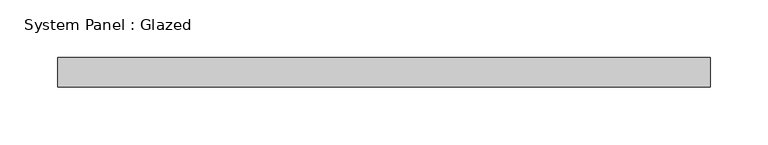
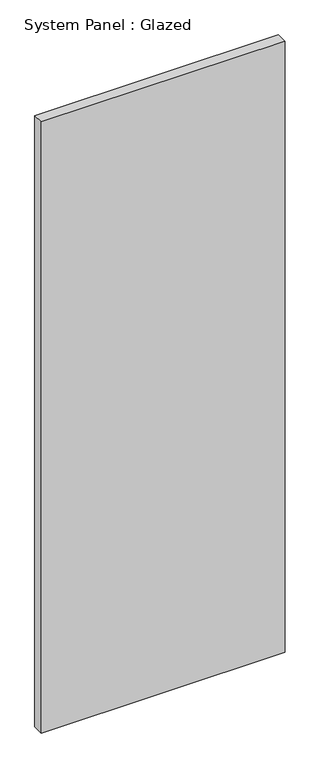
"""IFC4 building model written with IfcOpenShell, lengths in millimetres: plate geometry, System Panel : Glazed."""

from ifc_helpers import new_model, si_unit, origin, origin_with_axes, place, context, project, spatial, polyline, outline, extrude, source, transform, mapped, element, save


def system_panel_glazed_a47e91a8(model_context):
    return source(origin(), model_context, "Body", "SweptSolid", [
        extrude(outline(polyline([(282.575, 19.05), (-282.575, 19.05), (-282.575, 44.45), (282.575, 44.45), (282.575, 19.05)])), origin_with_axes(), (0.0, 0.0, 1.0), 1497.1102394),
    ])


if __name__ == "__main__":
    model = new_model("IFC4")
    model_context = context("Model", 3, world=origin())
    ifc_project = project(units=[si_unit("LENGTHUNIT", "METRE", prefix="MILLI")], contexts=[model_context])
    site = spatial("IfcSite", under=ifc_project)
    building = spatial("IfcBuilding", under=site)
    placement = place(None, origin())
    system_panel_glazed_shape = system_panel_glazed_a47e91a8(model_context)
    element("IfcPlate", 1, ObjectType="System Panel : Glazed", at=placement, inside=building, context=model_context, shape_type="MappedRepresentation", body=[
        mapped(system_panel_glazed_shape, transform((0.0, 0.0, 0.0), x_axis=(1.0, 0.0, 0.0), y_axis=(0.0, 1.0, 0.0), z_axis=(0.0, 0.0, 1.0))),
    ])
    save(model, "model.ifc")

# Revit data of these elements
# Type "System Panel : Glazed"
#   Construction Type Id = "GSP4R"
#   Analytic Construction = "1/8 in Pilkington single glazing"
#   Visual Light Transmittance = 0.9
#   Solar Heat Gain Coefficient = 0.86
#   Heat Transfer Coefficient (U) = 1.18115 BTU/(h·ft²·°F)
#   Define Thermal Properties by = 1
# Element 1 (IfcPlate, "System Panel : Glazed")
#   Materials on its faces: "Glass"
# Materials
#   "Glass": class "Glass", colour RGB 0 128 192, transparency 0.75, Description = "Soda Lime Glass", Cost = 0
